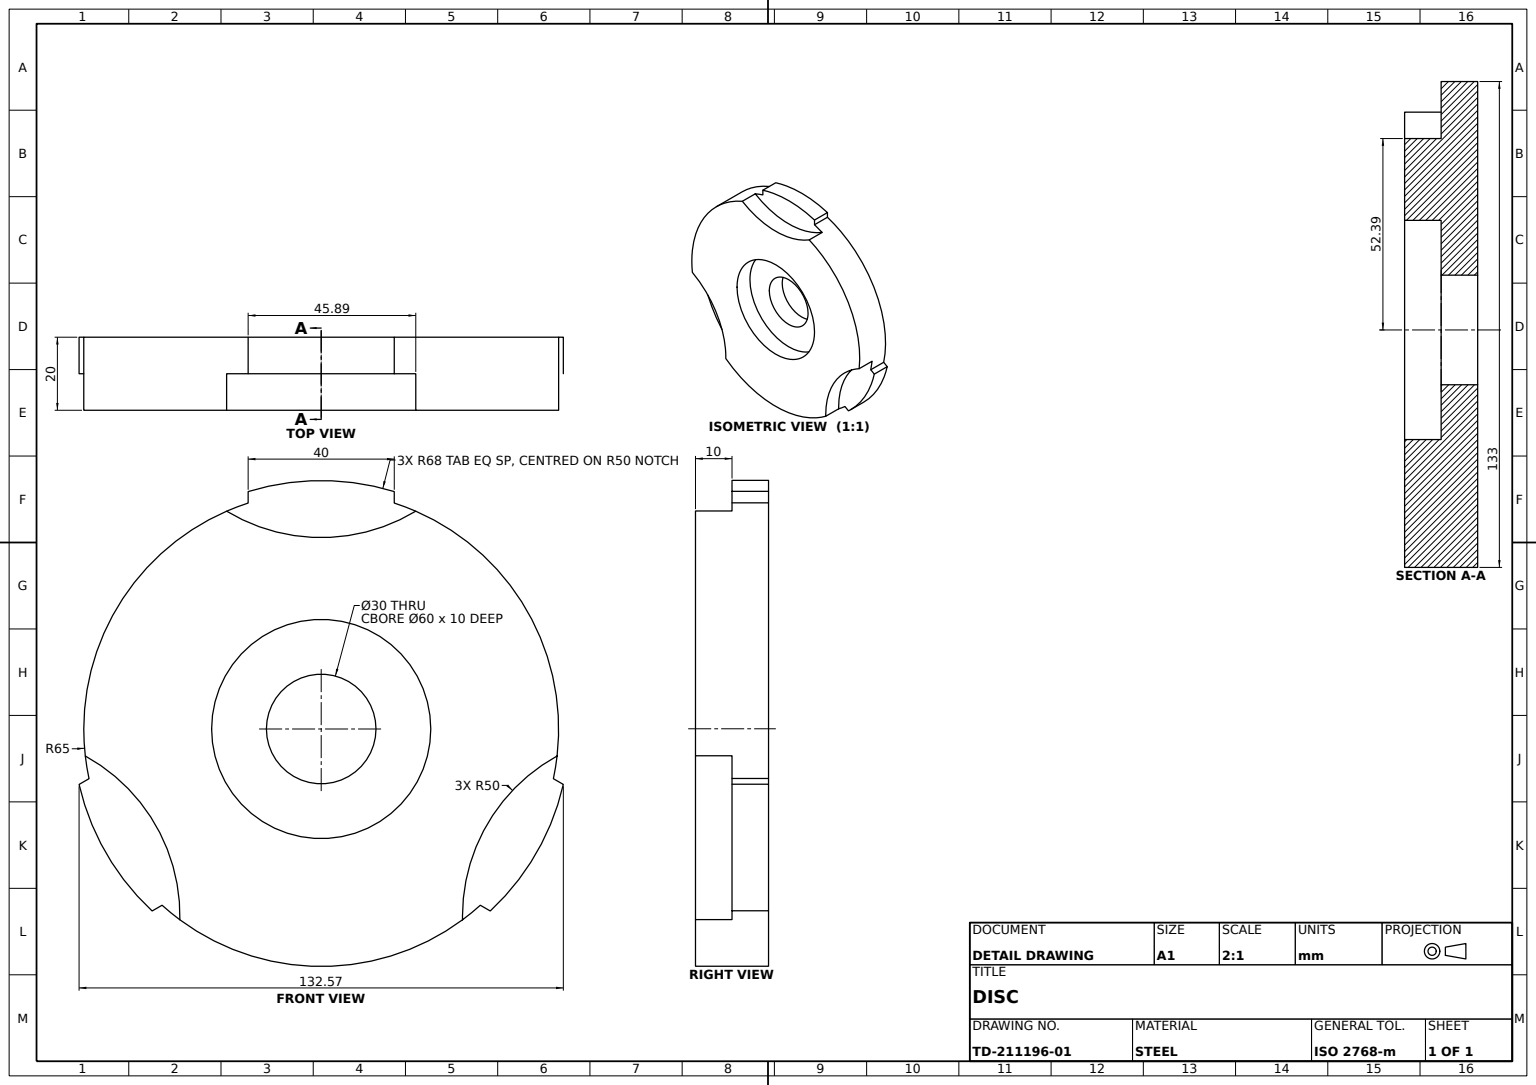
from build123d import *

# Parameters (mm, degrees)
BASE_DISC_DEPTH       = 10
UPPER_SECTION_DEPTH   = 10
COUNTERBORE_SKETCH_R  = 30
COUNTERBORE_DEPTH     = 10
THROUGH_BORE_SKETCH_R = 15
THROUGH_BORE_DEPTH    = 10


with BuildPart() as part:
    # Base Disc Profile Sketch → Base Disc (new body)
    with BuildSketch(Plane.XY):
        with BuildLine():
            Line((20, 61.846584384), (20, 64.992307237))
            ThreePointArc((20, 64.992307237), (0, 68), (-20, 64.992307237))
            Line((-20, 64.992307237), (-20, 61.846584384))
            ThreePointArc((-20, 61.846584384), (-56.291651246, 32.5), (-63.560713214, -13.602784116))
            Line((-63.560713214, -13.602784116), (-66.284989118, -15.175645543))
            ThreePointArc((-66.284989118, -15.175645543), (-58.889727457, -34), (-46.284989118, -49.816661694))
            Line((-46.284989118, -49.816661694), (-43.560713214, -48.243800268))
            ThreePointArc((-43.560713214, -48.243800268), (0, -65), (43.560713214, -48.243800268))
            Line((43.560713214, -48.243800268), (46.284989118, -49.816661694))
            ThreePointArc((46.284989118, -49.816661694), (58.889727457, -34), (66.284989118, -15.175645543))
            Line((66.284989118, -15.175645543), (63.560713214, -13.602784116))
            ThreePointArc((63.560713214, -13.602784116), (56.291651246, 32.5), (20, 61.846584384))
        make_face()
    extrude(amount=BASE_DISC_DEPTH)

    # Upper Section Sketch → Upper Section (add)
    with BuildSketch(Plane.XY.offset(10)):
        with BuildLine():
            ThreePointArc((-25.892074701, 59.620470207), (-56.291651246, 32.5), (-64.578879135, -7.387040655))
            ThreePointArc((-64.578879135, -7.387040655), (-45.374794332, -26.197149722), (-38.686804434, -52.233429551))
            ThreePointArc((-38.686804434, -52.233429551), (0, -65), (38.686804434, -52.233429551))
            ThreePointArc((38.686804434, -52.233429551), (45.374794332, -26.197149722), (64.578879135, -7.387040655))
            ThreePointArc((64.578879135, -7.387040655), (56.291651246, 32.5), (25.892074701, 59.620470207))
            ThreePointArc((25.892074701, 59.620470207), (0, 52.394299444), (-25.892074701, 59.620470207))
        make_face()
    extrude(amount=UPPER_SECTION_DEPTH)

    # Counterbore Sketch → Counterbore (cut)
    with BuildSketch(Plane.XY.offset(20)):
        Circle(COUNTERBORE_SKETCH_R)
    extrude(amount=-COUNTERBORE_DEPTH, mode=Mode.SUBTRACT)

    # Through Bore Sketch → Through Bore (cut)
    with BuildSketch(Plane.XY.offset(10)):
        Circle(THROUGH_BORE_SKETCH_R)
    extrude(amount=-THROUGH_BORE_DEPTH, mode=Mode.SUBTRACT)


solid = part.part
